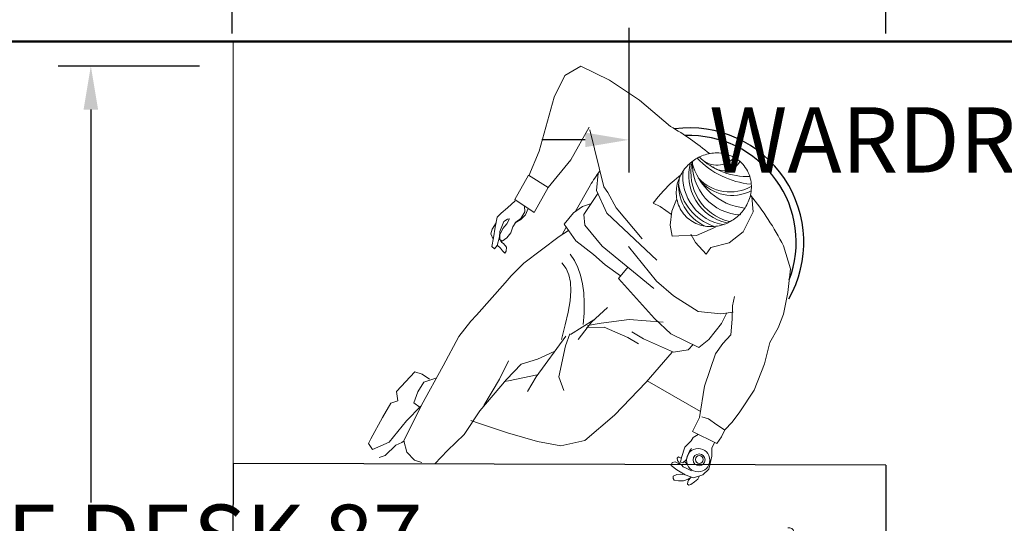
# Model space of a CAD drawing. Units: inches. Extents: x -466983 to 1020, y 324 to 318697.
# Tile 39 of 97: x 817 to 908, y 781 to 827. Entities that reach past the tile are written whole.
import ezdxf

# ---------------------------------------------------------------- set-up
doc = ezdxf.new("R2010")
doc.units = ezdxf.units.IN
doc.header["$MEASUREMENT"] = 0
for name, color, linetype, lineweight in [('A-ANNO-DIMS', 2, 'Continuous', 18), ('A-FLOR-PATT', 252, 'Continuous', 13), ('A-FURN', 8, 'Continuous', 18), ('A-WALL', 7, 'Continuous', 50), ('CBV_01', 7, 'Continuous', 0)]:
    doc.layers.add(name, color=color, linetype=linetype, lineweight=lineweight)
doc.layers.add('Office Desk', color=30, linetype='Continuous', true_color=0xeb7500)
doc.styles.get("Standard").update_dxf_attribs({"font": 'arial.ttf'})
doc.dimstyles.get("Standard").update_dxf_attribs({"dimtxt": 6, "dimasz": 4, "dimexe": 3, "dimexo": 3, "dimgap": 0.09, "dimtad": 0, "dimtih": 1, "dimtoh": 1, "dimdec": 1, "dimzin": 0, "dimdsep": 46, "dimlunit": 3, "dimtxsty": 'Standard', "dimcen": 0.09, "dimadec": 0, "dimazin": 0, "dimtfac": 1, "dimtdec": 1, "dimtofl": 0, "dimtmove": 0, "dimatfit": 3, "dimfxl": 1, "dimtolj": 1, "dimtzin": 0, "dimarcsym": 0})

# ---------------------------------------------------------------- blocks, each defined once
blk = doc.blocks.new('Offce Table')
at = {"layer": 'CBV_01'}
h = blk.add_hatch(dxfattribs=at)
h.set_pattern_fill('HEX', color=256, scale=1.206041, angle=-45.15377, style=0)
h.set_pattern_definition([(44.846232, (2370.5468, 299.66597), (0.18414034, -0.18513138), [0.1507551, -0.30151019]), (284.846232, (2370.5468, 299.66597), (-0.25239865, -0.06690453), [0.1507551, -0.30151019]), (344.846232, (2370.6537, 299.77229), (-0.06825831, -0.25203591), [0.1507551, -0.30151019])])
h.paths.add_polyline_path([(2601.472, 956.599), (2601.473, 957.136, -4.924372), (2599.622, 957.141), (2599.621, 956.604, 3.823416)])
for p, q in [((2608.415, 1012.503, -0.016), (2606.746, 1009.522, -0.016)), ((2609.784, 1007.023, -0.016), (2608.49, 1012.271, -0.016)), ((2606.746, 1009.522, -0.016), (2604.659, 1006.977, -0.016)), ((2609.256, 1008.271, -0.016), (2609.109, 1006.706, -0.016)), ((2602.849, 1008.103, -0.016), (2601.613, 1005.868, -0.016)), ((2604.659, 1006.977, -0.016), (2602.849, 1008.103, -0.016)), ((2604.659, 1006.977, -0.016), (2603.369, 1004.683, -0.016)), ((2607.133, 1004.729, -0.016), (2608.517, 1007.151, -0.016)), ((2609.109, 1006.706, -0.016), (2610.057, 1004.601, -0.016)), ((2603.369, 1004.683, -0.016), (2601.613, 1005.868, -0.016)), ((2610.057, 1004.601, -0.016), (2614.644, 1000.305, -0.016)), ((2605.941, 1002.644, -0.016), (2606.327, 1003.319, -0.016)), ((2612.11, 994.853, -0.016), (2609.52, 994.501, -0.016)), ((2615.216, 994.607, -0.016), (2612.11, 994.853, -0.016)), ((2609.52, 994.501, -0.016), (2608.271, 994.303, -0.016)), ((2618.647, 986.395, -0.016), (2613.748, 989.194, -0.016)), ((2625.938, 974.583, -0.016), (2624.545, 974.304, -0.016)), ((2626.476, 972.945, -0.016), (2617.003, 972.971, -0.016)), ((2616.528, 972.498, -0.016), (2616.499, 961.604, -0.016)), ((2617.001, 972.023, -0.016), (2616.976, 963.024, -0.016)), ((2622.832, 972.481, -0.016), (2617.475, 972.496, -0.016)), ((2622.49, 972.008, -0.016), (2617.948, 972.021, -0.016)), ((2626.001, 972.473, -0.016), (2622.97, 972.481, -0.016)), ((2625.552, 972, -0.016), (2623.065, 972.007, -0.016)), ((2623.609, 963.48, -0.016), (2623.632, 972.005, -0.016)), ((2626.919, 961.576, -0.016), (2626.948, 972.47, -0.016)), ((2590.067, 965.862, -0.016), (2590.368, 971.161, -0.016)), ((2590.877, 971.137, -0.016), (2603.66, 971.102, -0.016)), ((2591.166, 971.955, -0.016), (2608.412, 971.908, -0.016)), ((2591.557, 971.135, -0.016), (2591.555, 970.498, -0.016)), ((2592.439, 971.132, -0.016), (2592.437, 970.496, -0.016)), ((2593.31, 971.13, -0.016), (2593.309, 970.493, -0.016)), ((2600.28, 971.111, -0.016), (2600.278, 970.474, -0.016)), ((2601.151, 971.109, -0.016), (2601.15, 970.472, -0.016)), ((2602.023, 971.107, -0.016), (2602.021, 970.47, -0.016)), ((2602.894, 971.104, -0.016), (2602.892, 970.467, -0.016)), ((2604.302, 971.1, -0.016), (2606.269, 971.095, -0.016)), ((2609.478, 965.81, -0.016), (2609.206, 971.11, -0.016)), ((2617.473, 971.548, -0.016), (2617.451, 963.496, -0.016)), ((2622.661, 963.482, -0.016), (2622.684, 971.877, -0.016)), ((2625.977, 963.473, -0.016), (2625.998, 971.525, -0.016)), ((2626.449, 962.998, -0.016), (2626.473, 971.998, -0.016)), ((2590.761, 970.595, -0.016), (2590.787, 971.051, -0.016)), ((2590.827, 970.256, -0.016), (2603.657, 970.221, -0.016)), ((2590.851, 970.5, -0.016), (2603.658, 970.465, -0.016)), ((2592.1, 970.252, -0.016), (2592.098, 969.616, -0.016)), ((2592.971, 970.25, -0.016), (2592.97, 969.613, -0.016)), ((2593.842, 970.248, -0.016), (2593.841, 969.611, -0.016)), ((2594.714, 970.245, -0.016), (2594.712, 969.609, -0.016)), ((2595.585, 970.243, -0.016), (2595.583, 969.606, -0.016)), ((2596.456, 970.241, -0.016), (2596.454, 969.604, -0.016)), ((2597.327, 970.238, -0.016), (2597.326, 969.602, -0.016)), ((2598.199, 970.236, -0.016), (2598.197, 969.599, -0.016)), ((2599.07, 970.234, -0.016), (2599.068, 969.597, -0.016)), ((2599.941, 970.231, -0.016), (2599.939, 969.595, -0.016)), ((2600.812, 970.229, -0.016), (2600.811, 969.592, -0.016)), ((2601.683, 970.227, -0.016), (2601.682, 969.59, -0.016)), ((2603.75, 971.012, -0.016), (2603.749, 970.555, -0.016)), ((2604.211, 971.011, -0.016), (2604.21, 970.554, -0.016)), ((2604.3, 970.464, -0.016), (2606.267, 970.458, -0.016)), ((2604.928, 971.099, -0.016), (2604.926, 970.462, -0.016)), ((2605.015, 970.218, -0.016), (2605.551, 970.216, -0.016)), ((2605.643, 971.097, -0.016), (2605.642, 970.46, -0.016)), ((2606.359, 971.005, -0.016), (2606.358, 970.548, -0.016)), ((2606.821, 971.004, -0.016), (2606.82, 970.547, -0.016)), ((2606.909, 970.213, -0.016), (2608.289, 970.209, -0.016)), ((2606.91, 970.457, -0.016), (2608.29, 970.453, -0.016)), ((2606.911, 971.093, -0.016), (2608.697, 971.089, -0.016)), ((2607.309, 970.212, -0.016), (2607.307, 969.575, -0.016)), ((2607.311, 971.092, -0.016), (2607.31, 970.456, -0.016)), ((2607.799, 970.21, -0.016), (2607.798, 969.573, -0.016)), ((2607.802, 971.091, -0.016), (2607.8, 970.454, -0.016)), ((2608.292, 971.09, -0.016), (2608.288, 969.572, -0.016)), ((2608.855, 969.666, -0.016), (2608.787, 971.003, -0.016)), ((2590.711, 969.714, -0.016), (2590.737, 970.171, -0.016)), ((2590.777, 969.375, -0.016), (2603.655, 969.34, -0.016)), ((2590.801, 969.619, -0.016), (2603.656, 969.585, -0.016)), ((2591.215, 969.374, -0.016), (2591.214, 968.737, -0.016)), ((2592.098, 969.371, -0.016), (2592.096, 968.735, -0.016)), ((2592.969, 969.369, -0.016), (2592.967, 968.732, -0.016)), ((2593.84, 969.367, -0.016), (2593.838, 968.73, -0.016)), ((2594.711, 969.364, -0.016), (2594.71, 968.728, -0.016)), ((2595.583, 969.362, -0.016), (2595.581, 968.725, -0.016)), ((2596.454, 969.36, -0.016), (2596.452, 968.723, -0.016)), ((2597.325, 969.357, -0.016), (2597.323, 968.721, -0.016)), ((2598.196, 969.355, -0.016), (2598.195, 968.718, -0.016)), ((2599.067, 969.353, -0.016), (2599.066, 968.716, -0.016)), ((2599.939, 969.35, -0.016), (2599.937, 968.714, -0.016)), ((2600.81, 969.348, -0.016), (2600.808, 968.711, -0.016)), ((2601.681, 969.346, -0.016), (2601.679, 968.709, -0.016)), ((2602.552, 969.343, -0.016), (2602.55, 968.463, -0.016)), ((2603.747, 970.131, -0.016), (2603.746, 969.675, -0.016)), ((2604.925, 970.128, -0.016), (2604.924, 969.671, -0.016)), ((2605.014, 969.581, -0.016), (2605.549, 969.579, -0.016)), ((2605.641, 970.126, -0.016), (2605.64, 969.669, -0.016)), ((2606.818, 970.123, -0.016), (2606.817, 969.666, -0.016)), ((2606.907, 969.576, -0.016), (2608.765, 969.571, -0.016)), ((2606.907, 969.332, -0.016), (2608.787, 969.327, -0.016)), ((2607.307, 969.331, -0.016), (2607.305, 968.694, -0.016)), ((2607.797, 969.329, -0.016), (2607.795, 968.693, -0.016)), ((2608.287, 969.328, -0.016), (2608.283, 967.81, -0.016)), ((2590.611, 967.953, -0.016), (2590.637, 968.409, -0.016)), ((2590.661, 968.834, -0.016), (2590.687, 969.29, -0.016)), ((2590.727, 968.494, -0.016), (2602.55, 968.463, -0.016)), ((2590.751, 968.738, -0.016), (2602.551, 968.707, -0.016)), ((2591.751, 968.491, -0.016), (2591.75, 967.855, -0.016)), ((2592.623, 968.489, -0.016), (2592.621, 967.852, -0.016)), ((2593.494, 968.487, -0.016), (2593.492, 967.85, -0.016)), ((2594.365, 968.484, -0.016), (2594.363, 967.848, -0.016)), ((2595.236, 968.482, -0.016), (2595.235, 967.845, -0.016)), ((2596.108, 968.48, -0.016), (2596.106, 967.843, -0.016)), ((2596.979, 968.477, -0.016), (2596.977, 967.841, -0.016)), ((2597.85, 968.475, -0.016), (2597.848, 967.838, -0.016)), ((2598.721, 968.473, -0.016), (2598.719, 967.836, -0.016)), ((2599.592, 968.47, -0.016), (2599.591, 967.834, -0.016)), ((2600.464, 968.468, -0.016), (2600.462, 967.831, -0.016)), ((2601.335, 968.466, -0.016), (2601.333, 967.829, -0.016)), ((2602.092, 968.464, -0.016), (2602.091, 967.827, -0.016)), ((2603.745, 969.25, -0.016), (2603.741, 967.913, -0.016)), ((2604.295, 968.458, -0.016), (2606.262, 968.453, -0.016)), ((2604.92, 968.456, -0.016), (2604.919, 967.819, -0.016)), ((2605.636, 968.454, -0.016), (2605.635, 967.817, -0.016)), ((2606.816, 969.242, -0.016), (2606.815, 968.785, -0.016)), ((2606.904, 968.451, -0.016), (2608.285, 968.447, -0.016)), ((2606.905, 968.695, -0.016), (2608.285, 968.691, -0.016)), ((2607.304, 968.45, -0.016), (2607.303, 967.813, -0.016)), ((2607.794, 968.448, -0.016), (2607.793, 967.812, -0.016)), ((2608.946, 967.904, -0.016), (2608.877, 969.241, -0.016)), ((2590.561, 967.072, -0.016), (2590.587, 967.528, -0.016)), ((2590.677, 967.613, -0.016), (2603.65, 967.579, -0.016)), ((2590.701, 967.858, -0.016), (2603.651, 967.823, -0.016)), ((2591.526, 967.611, -0.016), (2591.525, 966.974, -0.016)), ((2592.409, 967.609, -0.016), (2592.407, 966.972, -0.016)), ((2593.28, 967.606, -0.016), (2593.278, 966.97, -0.016)), ((2594.151, 967.604, -0.016), (2594.149, 966.967, -0.016)), ((2595.022, 967.602, -0.016), (2595.021, 966.965, -0.016)), ((2595.893, 967.599, -0.016), (2595.892, 966.963, -0.016)), ((2596.765, 967.597, -0.016), (2596.763, 966.96, -0.016)), ((2597.636, 967.595, -0.016), (2597.634, 966.958, -0.016)), ((2598.507, 967.592, -0.016), (2598.505, 966.956, -0.016)), ((2599.378, 967.59, -0.016), (2599.377, 966.953, -0.016)), ((2600.25, 967.588, -0.016), (2600.248, 966.951, -0.016)), ((2601.121, 967.585, -0.016), (2601.119, 966.949, -0.016)), ((2601.992, 967.583, -0.016), (2601.99, 966.946, -0.016)), ((2602.863, 967.581, -0.016), (2602.862, 966.944, -0.016)), ((2603.74, 967.488, -0.016), (2603.739, 967.032, -0.016)), ((2604.202, 967.487, -0.016), (2604.201, 967.031, -0.016)), ((2604.204, 968.368, -0.016), (2604.203, 967.911, -0.016)), ((2604.292, 967.577, -0.016), (2606.26, 967.572, -0.016)), ((2604.293, 967.821, -0.016), (2606.26, 967.816, -0.016)), ((2604.918, 967.575, -0.016), (2604.916, 966.938, -0.016)), ((2605.634, 967.573, -0.016), (2605.632, 966.937, -0.016)), ((2606.352, 968.362, -0.016), (2606.351, 967.906, -0.016)), ((2606.814, 968.361, -0.016), (2606.813, 967.904, -0.016)), ((2606.902, 967.814, -0.016), (2608.855, 967.809, -0.016)), ((2606.902, 967.57, -0.016), (2608.878, 967.565, -0.016)), ((2607.302, 967.569, -0.016), (2607.3, 966.932, -0.016)), ((2607.792, 967.568, -0.016), (2607.79, 966.931, -0.016)), ((2608.282, 967.566, -0.016), (2608.281, 966.929, -0.016)), ((2610.991, 968.125, -0.016), (2610.989, 967.24, -0.016)), ((2613.126, 967.234, -0.016), (2613.129, 968.12, -0.016)), ((2618.946, 967.738, -0.016), (2618.938, 964.699, -0.016)), ((2621.142, 967.732, -0.016), (2618.946, 967.738, -0.016)), ((2621.134, 964.693, -0.016), (2621.142, 967.732, -0.016)), ((2590.651, 966.977, -0.016), (2603.649, 966.942, -0.016)), ((2604.291, 966.94, -0.016), (2606.258, 966.935, -0.016)), ((2606.35, 967.481, -0.016), (2606.348, 967.025, -0.016)), ((2606.811, 967.48, -0.016), (2606.81, 967.024, -0.016)), ((2606.9, 966.933, -0.016), (2608.901, 966.928, -0.016)), ((2608.991, 967.023, -0.016), (2608.968, 967.479, -0.016)), ((2590.463, 965.974, -0.016), (2590.489, 966.43, -0.016)), ((2590.553, 965.879, -0.016), (2603.646, 965.843, -0.016)), ((2590.579, 966.515, -0.016), (2603.647, 966.48, -0.016)), ((2591.208, 966.514, -0.016), (2591.206, 965.877, -0.016)), ((2592.09, 966.511, -0.016), (2592.088, 965.874, -0.016)), ((2592.961, 966.509, -0.016), (2592.959, 965.872, -0.016)), ((2593.832, 966.507, -0.016), (2593.831, 965.87, -0.016)), ((2594.704, 966.504, -0.016), (2594.702, 965.867, -0.016)), ((2595.575, 966.502, -0.016), (2595.573, 965.865, -0.016)), ((2596.446, 966.5, -0.016), (2596.444, 965.863, -0.016)), ((2597.317, 966.497, -0.016), (2597.316, 965.86, -0.016)), ((2598.189, 966.495, -0.016), (2598.187, 965.858, -0.016)), ((2599.06, 966.493, -0.016), (2599.058, 965.856, -0.016)), ((2599.931, 966.49, -0.016), (2599.929, 965.853, -0.016)), ((2600.802, 966.488, -0.016), (2600.8, 965.851, -0.016)), ((2601.673, 966.485, -0.016), (2601.672, 965.849, -0.016)), ((2602.545, 966.483, -0.016), (2602.543, 965.846, -0.016)), ((2603.737, 966.39, -0.016), (2603.736, 965.933, -0.016)), ((2604.199, 966.389, -0.016), (2604.198, 965.932, -0.016)), ((2604.288, 965.842, -0.016), (2606.255, 965.836, -0.016)), ((2604.289, 966.478, -0.016), (2606.257, 966.473, -0.016)), ((2604.915, 966.477, -0.016), (2604.913, 965.84, -0.016)), ((2605.631, 966.475, -0.016), (2605.629, 965.838, -0.016)), ((2606.347, 966.383, -0.016), (2606.346, 965.926, -0.016)), ((2591.651, 963.61, -0.016), (2591.652, 964.18, -0.016)), ((2591.652, 964.18, -0.016), (2607.884, 964.136, -0.016)), ((2607.883, 963.567, -0.016), (2607.884, 964.136, -0.016)), ((2618.938, 964.699, -0.016), (2621.134, 964.693, -0.016)), ((2591.651, 963.61, -0.016), (2607.883, 963.567, -0.016)), ((2617.924, 963.021, -0.016), (2622.186, 963.01, -0.016)), ((2624.081, 963.005, -0.016), (2625.502, 963.001, -0.016)), ((2617.449, 962.549, -0.016), (2625.974, 962.526, -0.016)), ((2616.971, 961.129, -0.016), (2626.444, 961.104, -0.016)), ((2587.523, 957.485, -0.016), (2587.529, 959.809, -0.016)), ((2588.012, 959.808, -0.016), (2587.529, 959.809, -0.016)), ((2588.008, 958.361, -0.016), (2588.012, 959.808, -0.016)), ((2613.097, 959.741, -0.016), (2588.012, 959.808, -0.016)), ((2613.093, 958.293, -0.016), (2613.097, 959.741, -0.016)), ((2613.097, 959.741, -0.016), (2613.58, 959.739, -0.016)), ((2613.574, 957.415, -0.016), (2613.58, 959.739, -0.016)), ((2613.575, 957.83, -0.016), (2587.524, 957.9, -0.016)), ((2613.093, 958.293, -0.016), (2588.008, 958.361, -0.016)), ((2613.574, 957.415, -0.016), (2587.523, 957.485, -0.016)), ((2599.623, 957.453, -0.016), (2599.616, 954.956, -0.016)), ((2601.467, 954.951, -0.016), (2601.474, 957.448, -0.016))]:
    blk.add_line(p, q, dxfattribs=at)
at = {"layer": 'CBV_01', "elevation": -0.016}
for points in [[(2615.905, 1012.577), (2613.053, 1014.982), (2610.299, 1016.845), (2607.657, 1018.131), (2606.194, 1017.275), (2605.217, 1015.268), (2603.853, 1010.314), (2602.879, 1008.045)], [(2615.988, 1004.478), (2614.96, 1005.208), (2614.308, 1005.525), (2614.757, 1006.113), (2615.264, 1006.672), (2615.861, 1007.303), (2616.828, 1008.098)], [(2609.237, 1006.422), (2607.928, 1004.486), (2608.031, 1003.515), (2609.627, 1001.587), (2614.38, 997.692)], [(2609.784, 1007.023), (2610.157, 1006.5), (2610.923, 1005.091), (2613.301, 1002.25)], [(2601.645, 1005.757), (2600.928, 1005.093), (2600.35, 1004.604), (2599.991, 1004.244), (2599.803, 1003.315), (2599.638, 1002.347), (2599.483, 1001.54), (2599.724, 1001.344), (2599.967, 1001.637), (2600.182, 1002.428), (2600.223, 1002.939), (2600.601, 1003.849), (2600.919, 1004.057), (2601.126, 1004.099), (2600.864, 1003.615), (2600.488, 1003.194), (2600.232, 1002.61), (2600.215, 1002.19), (2600.434, 1002.033), (2600.876, 1002.337), (2601.229, 1002.797), (2601.417, 1003.366), (2601.693, 1003.781), (2602.143, 1004.116), (2602.508, 1004.736), (2602.488, 1005.264)], [(2611.311, 998.838), (2609.891, 999.854), (2608.816, 1000.825), (2607.213, 1002.053), (2606.132, 1003.597), (2607.005, 1004.637), (2607.817, 1005.219), (2608.551, 1005.472)], [(2620.03, 1003.316), (2618.279, 1002.557), (2616.657, 1002.54), (2616.056, 1002.487), (2615.859, 1003.504), (2616.03, 1004.802), (2616.435, 1005.872)], [(2623.369, 1006.108), (2623.489, 1004.742), (2622.583, 1002.88), (2621.297, 1001.894), (2619.588, 1001.46), (2619.177, 1000.853), (2618.193, 1001.908), (2617.768, 1002.691)], [(2602.82, 1005.043), (2602.594, 1004.451), (2602.149, 1004.017), (2601.646, 1003.729)], [(2599.88, 1003.719), (2599.524, 1003.13), (2599.408, 1002.704), (2599.605, 1002.226)], [(2606.528, 1003.032), (2605.68, 1002.471), (2602.418, 1000.03), (2601.273, 998.86), (2600.724, 998.206)], [(2599.975, 1001.667), (2600.29, 1001.386), (2600.484, 1001.137), (2600.694, 1000.949), (2600.805, 1001.115), (2600.843, 1001.497), (2600.575, 1001.831), (2600.401, 1001.911), (2600.29, 1002.105)], [(2621.645, 995.508), (2620.535, 995.357), (2618.448, 995.567), (2616.162, 997.025), (2614.619, 998.351), (2612.039, 1001.547)], [(2626.275, 1001.616), (2626.928, 999.499), (2626.674, 997.32), (2626.279, 995.325), (2625.783, 994.07), (2625.011, 992.719), (2624.523, 990.769), (2623.577, 988.351), (2622.255, 986.346), (2621.571, 985.413), (2620.884, 984.711), (2620.567, 984.06), (2620.156, 983.454), (2617.921, 984.542), (2618.555, 985.845), (2619.033, 988.72), (2620.019, 991.694), (2620.704, 992.627), (2621.436, 993.422), (2621.56, 994.859), (2621.592, 996.109), (2621.768, 996.945)], [(2621.045, 995.403), (2620.596, 994.482), (2619.433, 993.012), (2618.508, 992.282), (2615.939, 993.532), (2614.417, 994.924), (2611.117, 998.606), (2612.006, 999.68)], [(2598.079, 995.226), (2600.724, 998.206)], [(2610.106, 995.943), (2608.639, 994.585), (2607.406, 992.997)], [(2593.057, 981.705), (2592.391, 981.926), (2591.699, 982.654), (2591.425, 983.702), (2593.018, 986.977), (2595.029, 990.571), (2596.471, 993.266), (2597.559, 994.696), (2598.079, 995.226)], [(2608.868, 994.819), (2606.706, 993.453)], [(2612.969, 992.593), (2611.989, 993.184), (2609.802, 994.134), (2608.181, 994.117)], [(2606.3, 993.316), (2603.556, 989.557), (2602.782, 988.235)], [(2606.666, 993.53), (2606.258, 992.422), (2605.658, 989.579), (2606.092, 988.322)], [(2617.981, 992.539), (2617.509, 992.046), (2616.173, 991.839), (2613.427, 993.06), (2612.354, 993.697)], [(2616.041, 991.842), (2613.653, 989.084), (2610.743, 986.059), (2608.035, 983.719), (2605.833, 983.223), (2603.674, 983.62), (2600.931, 984.432), (2598.346, 985.299), (2597.555, 985.553)], [(2601.016, 991.054), (2600.194, 989.364), (2598.749, 986.932)], [(2602.176, 990.751), (2603.695, 991.187), (2605.212, 991.886)], [(2602.176, 990.751), (2600.825, 989.318), (2598.386, 986.455), (2596.938, 984.285), (2595.43, 982.798), (2594.268, 981.566)], [(2593.781, 989.349), (2593.092, 989.815), (2592.407, 990.018), (2590.745, 988.214), (2590.859, 987.374), (2590.231, 987.158), (2589.457, 985.836), (2588.374, 983.881), (2588.169, 983.458), (2588.543, 982.884), (2590.06, 983.583), (2591.668, 985.544), (2592.967, 986.871)], [(2594.358, 989.46), (2593.258, 989.081), (2592.69, 988.182), (2592.333, 987.18), (2592.916, 986.765)], [(2603.658, 989.768), (2602.347, 989.491), (2601.036, 989.215), (2600.616, 989.158)], [(2620.869, 984.711), (2620.142, 985.171), (2619.396, 985.724), (2618.764, 985.904)], [(2618.427, 984.285), (2617.992, 984.009), (2617.799, 983.689), (2617.455, 983.369), (2617.216, 983.109), (2616.915, 982.152), (2616.829, 981.743), (2617.026, 981.685), (2617.34, 981.945), (2617.643, 982.751), (2617.837, 982.995)], [(2589.13, 982.155), (2589.704, 982.337), (2590.671, 983.296), (2591.214, 983.532), (2591.428, 983.678)], [(2619.946, 983.546), (2619.695, 983.03), (2619.703, 982.275), (2619.429, 981.094), (2618.876, 980.574), (2618.018, 980.278), (2617.259, 980.573), (2616.468, 981.032), (2615.95, 981.435), (2616.038, 981.692), (2616.339, 981.771), (2616.582, 981.653), (2616.932, 981.445), (2617.054, 981.31), (2617.389, 981.148), (2617.632, 981.03), (2617.814, 980.941)], [(2616.879, 982.095), (2616.619, 982.222), (2616.509, 982.091), (2616.53, 981.897), (2616.727, 981.641), (2616.83, 981.522)], [(2617.45, 981.473), (2617.29, 981.711), (2617.159, 981.821)], [(2617.842, 980.339), (2617.529, 980.17), (2617.087, 980.017), (2616.633, 980.031), (2616.226, 980.091), (2616.132, 980.229), (2616.139, 980.433), (2616.479, 980.612), (2616.793, 980.643), (2616.96, 980.608), (2617.219, 980.62)], [(2618.571, 980.467), (2618.408, 980.179), (2618.096, 979.917), (2617.756, 979.691), (2617.581, 979.616), (2617.451, 979.725), (2617.476, 979.92), (2617.558, 980.087), (2617.731, 980.301)], [(2612.055, 966.169), (2611.856, 964.989), (2611.679, 963.716), (2611.02, 962.076), (2610.22, 960.793), (2609.486, 959.75)], [(2606.891, 963.569), (2606.795, 962.987), (2606.508, 962.105), (2606.218, 960.599), (2605.987, 959.76)], [(2605.259, 957.437), (2604.573, 956.5), (2603.741, 956.009), (2602.914, 954.947)], [(2607.854, 957.43), (2607.669, 957.168), (2607.117, 956.845), (2606.434, 956.343), (2605.915, 956.117), (2604.644, 955.241), (2604.076, 954.87), (2602.914, 954.897)]]:
    blk.add_lwpolyline(points, dxfattribs=at)
blk.add_lwpolyline([(2617.847, 1009.329, -0.080167), (2618.927, 1009.931, -0.088923), (2620.168, 1010.146, -0.104957), (2621.517, 1009.851, -0.120011), (2622.66, 1008.958, -0.120011), (2623.265, 1007.64, -0.104957), (2623.24, 1006.259, -0.088923), (2622.744, 1005.101, -0.080167), (2621.908, 1004.19, -0.080167), (2620.828, 1003.587, -0.088923), (2619.587, 1003.373, -0.104957), (2618.238, 1003.667, -0.120011), (2617.095, 1004.56, -0.120011), (2616.491, 1005.879, -0.104957), (2616.516, 1007.26, -0.088923), (2617.012, 1008.417, -0.080167)], format="xyb", close=True, dxfattribs=at)
at = {"layer": 'CBV_01'}
for points in [[(2605.883, 992.996), (2606.24, 994.337), (2606.508, 995.522), (2606.681, 996.562), (2606.754, 997.472), (2606.719, 998.261), (2606.572, 998.944), (2606.304, 999.532), (2605.911, 1000.037)], [(2607.865, 994.383), (2607.958, 995.416), (2607.981, 996.384), (2607.937, 997.288), (2607.824, 998.126), (2607.643, 998.9), (2607.394, 999.61), (2607.076, 1000.254), (2606.691, 1000.834)]]:
    blk.add_lwpolyline(points, dxfattribs=at)
at = {"layer": 'CBV_01', "elevation": -0.016}
for points in [[(2622.965, 972.508), (2622.413, 972.397), (2622.523, 971.845), (2623.075, 971.955)], [(2618.41, 970.567), (2617.848, 970.568), (2617.846, 970.005), (2618.409, 970.004)], [(2619.358, 970.564), (2618.795, 970.566), (2618.794, 970.003), (2619.356, 970.001)], [(2620.305, 970.562), (2619.742, 970.563), (2619.741, 970), (2620.304, 969.999)], [(2621.252, 970.559), (2620.69, 970.561), (2620.688, 969.998), (2621.251, 969.996)], [(2618.408, 969.54), (2617.845, 969.541), (2617.843, 968.978), (2618.406, 968.977)], [(2619.355, 969.537), (2618.792, 969.539), (2618.791, 968.976), (2619.353, 968.974)], [(2620.302, 969.535), (2619.74, 969.536), (2619.738, 968.973), (2620.301, 968.972)], [(2621.25, 969.532), (2620.687, 969.534), (2620.685, 968.971), (2621.248, 968.969)], [(2622.197, 969.53), (2621.634, 969.531), (2621.633, 968.968), (2622.195, 968.967)], [(2619.597, 967.597), (2619.034, 967.599), (2619.032, 967.036), (2619.595, 967.034)], [(2620.292, 967.595), (2619.73, 967.597), (2619.728, 967.034), (2620.291, 967.032)], [(2620.988, 967.594), (2620.425, 967.595), (2620.424, 967.032), (2620.986, 967.031)], [(2619.595, 966.902), (2619.032, 966.904), (2619.031, 966.341), (2619.593, 966.339)], [(2620.29, 966.9), (2619.728, 966.902), (2619.726, 966.339), (2620.289, 966.337)], [(2620.986, 966.898), (2620.423, 966.9), (2620.422, 966.337), (2620.985, 966.335)], [(2619.593, 966.207), (2619.03, 966.208), (2619.029, 965.645), (2619.591, 965.644)], [(2620.289, 966.205), (2619.726, 966.207), (2619.724, 965.643), (2620.287, 965.642)], [(2620.984, 966.203), (2620.422, 966.205), (2620.42, 965.642), (2620.983, 965.64)], [(2619.591, 965.475), (2619.028, 965.477), (2619.027, 964.914), (2619.589, 964.912)], [(2620.287, 965.473), (2619.724, 965.475), (2619.722, 964.912), (2620.285, 964.91)], [(2620.982, 965.471), (2620.42, 965.473), (2620.418, 964.91), (2620.981, 964.908)], [(2624.959, 963.21), (2624.96, 963.66), (2624.678, 963.661), (2624.677, 963.211)]]:
    blk.add_lwpolyline(points, close=True, dxfattribs=at)
at = {"layer": 'CBV_01', "const_width": 0.0942, "elevation": -0.016}
blk.add_lwpolyline([(2624.828, 963.196, -0.40574), (2623.816, 960.526, -1.618522), (2623.611, 961.83, -1.478802), (2622.602, 960.078, -0.24273), (2622.249, 961.227, -0.24273)], format="xyb", dxfattribs=at)
at = {"layer": 'CBV_01'}
for centre, radius in [((2618.438, 981.914, -0.016), 1.073), ((2618.528, 981.945, -0.016), 0.545), ((2618.543, 981.975, -0.016), 0.359), ((2607.595, 966.107, -0.016), 0.106), ((2608.057, 966.106, -0.016), 0.106), ((2608.519, 966.105, -0.016), 0.106), ((2594.113, 965.106, -0.016), 0.106), ((2594.575, 965.104, -0.016), 0.106), ((2595.037, 965.103, -0.016), 0.106), ((2595.499, 965.102, -0.016), 0.106), ((2595.961, 965.101, -0.016), 0.106), ((2596.423, 965.099, -0.016), 0.106), ((2596.885, 965.098, -0.016), 0.106)]:
    blk.add_circle(centre, radius, dxfattribs=at)
for centre, radius, start, end in [((2602.197, 989.221, -0.016), 27.082, 50.37515, 59.59099), ((2622.039, 1008.072, -0.016), 4.456, 164.47486, 257.30647), ((2622.408, 1008.336, -0.016), 4.634, 167.21461, 256.32515), ((2623.354, 1010.71, -0.016), 5.667, 194.03684, 263.23405), ((2622.533, 1009.067, -0.016), 4.614, 175.94557, 267.66665), ((2623.978, 1014.99, -0.016), 7.744, 223.41938, 264.68964), ((2622.956, 1014.334, -0.016), 6.357, 225.72213, 272.27484), ((2620.166, 1011.122, -0.016), 2.108, 227.18188, 318.83431), ((2620.826, 1010.16, -0.016), 1.655, 231.54376, 331.05244), ((2617.636, 1001.94, -0.016), 10.504, 141.43972, 150.25259), ((2621.493, 1007.946, -0.016), 4.465, 172.97935, 261.42536), ((2620.734, 1007.169, -0.016), 4.09, 171.47064, 246.35242), ((2621.463, 1008.017, -0.016), 4.872, 188.62106, 250.62094), ((2621.377, 1010.531, -0.016), 3.975, 222.55221, 299.84347), ((2621.553, 1010.092, -0.016), 3.854, 219.71778, 296.81649), ((2602.197, 989.221, -0.016), 27.082, 27.2384, 39.00595), ((2626.774, 975.233, -0.016), 0.474, 11.29645, 101.29645), ((2626.403, 974.675, -0.016), 0.474, 11.29645, 101.29645), ((2622.78, 973.469, -0.016), 0.474, 11.29645, 101.29645), ((2624.638, 973.84, -0.016), 0.474, 101.29645, 191.29645), ((2626.031, 974.118, -0.016), 0.474, 11.29645, 101.29645), ((2617.002, 972.497, -0.016), 0.474, 89.84532, 179.84532), ((2617.474, 972.022, -0.016), 0.474, 89.84532, 179.84532), ((2617.947, 971.547, -0.016), 0.474, 89.84532, 179.84532), ((2591.164, 971.159, -0.016), 0.796, 89.84623, 179.84623), ((2590.877, 971.046, -0.016), 0.0902, 89.84623, 176.75215), ((2603.66, 971.012, -0.016), 0.0902, 359.84623, 89.84623), ((2604.302, 971.01, -0.016), 0.0902, 89.84623, 179.84623), ((2608.41, 971.112, -0.016), 0.796, 359.84623, 89.84623), ((2590.827, 970.166, -0.016), 0.0902, 89.84623, 176.75215), ((2590.851, 970.59, -0.016), 0.0902, 176.75215, 269.84623), ((2603.657, 970.131, -0.016), 0.0902, 359.84623, 89.84623), ((2603.658, 970.556, -0.016), 0.0902, 269.84623, 359.84623), ((2604.3, 970.554, -0.016), 0.0902, 179.84623, 269.84623), ((2605.015, 970.127, -0.016), 0.0902, 89.84623, 179.84623), ((2605.551, 970.126, -0.016), 0.0902, 359.84623, 89.84623), ((2606.268, 970.549, -0.016), 0.0902, 269.84623, 359.84623), ((2606.269, 971.005, -0.016), 0.0902, 359.84623, 89.84623), ((2606.909, 970.122, -0.016), 0.0902, 89.84623, 179.84623), ((2606.91, 970.547, -0.016), 0.0902, 179.84623, 269.84623), ((2606.911, 971.003, -0.016), 0.0902, 89.84623, 179.84623), ((2608.696, 970.998, -0.016), 0.0902, 2.94029, 89.84623), ((2590.777, 969.285, -0.016), 0.0902, 89.84623, 176.75215), ((2590.801, 969.709, -0.016), 0.0902, 176.75215, 269.84623), ((2603.655, 969.25, -0.016), 0.0902, 359.84623, 89.84623), ((2603.656, 969.675, -0.016), 0.0902, 269.84623, 359.84623), ((2605.014, 969.671, -0.016), 0.0902, 179.84623, 269.84623), ((2605.549, 969.67, -0.016), 0.0902, 269.84623, 359.84623), ((2606.906, 969.241, -0.016), 0.0902, 89.84623, 179.84623), ((2606.907, 969.666, -0.016), 0.0902, 179.84623, 269.84623), ((2608.765, 969.661, -0.016), 0.0902, 269.84623, 2.94029), ((2608.787, 969.236, -0.016), 0.0902, 2.94029, 89.84623), ((2590.727, 968.404, -0.016), 0.0902, 89.84623, 176.75215), ((2590.751, 968.828, -0.016), 0.0902, 176.75215, 269.84623), ((2604.295, 968.368, -0.016), 0.0902, 89.84623, 179.84623), ((2606.262, 968.362, -0.016), 0.0902, 359.84623, 89.84623), ((2606.904, 968.361, -0.016), 0.0902, 89.84623, 179.84623), ((2606.905, 968.785, -0.016), 0.0902, 179.84623, 269.84623), ((2612.06, 968.122, -0.016), 1.069, 335.38444, 204.30803), ((2590.677, 967.523, -0.016), 0.0902, 89.84623, 176.75215), ((2590.701, 967.948, -0.016), 0.0902, 176.75215, 269.84623), ((2603.65, 967.488, -0.016), 0.0902, 359.84623, 89.84623), ((2603.651, 967.913, -0.016), 0.0902, 269.84623, 359.84623), ((2604.292, 967.487, -0.016), 0.0902, 89.84623, 179.84623), ((2604.293, 967.911, -0.016), 0.0902, 179.84623, 269.84623), ((2606.261, 967.906, -0.016), 0.0902, 269.84623, 359.84623), ((2606.259, 967.481, -0.016), 0.0902, 359.84623, 89.84623), ((2606.902, 967.48, -0.016), 0.0902, 89.84623, 179.84623), ((2606.903, 967.904, -0.016), 0.0902, 179.84623, 269.84623), ((2608.856, 967.899, -0.016), 0.0902, 269.84623, 2.94029), ((2608.877, 967.474, -0.016), 0.0902, 2.94029, 89.84623), ((2612.058, 967.237, -0.016), 1.069, 155.38444, 24.30803), ((2590.651, 967.067, -0.016), 0.0902, 176.75215, 269.84623), ((2603.649, 967.032, -0.016), 0.0902, 269.84623, 359.84623), ((2604.291, 967.03, -0.016), 0.0902, 179.84623, 269.84623), ((2606.258, 967.025, -0.016), 0.0902, 269.84623, 359.84623), ((2606.9, 967.023, -0.016), 0.0902, 179.84623, 269.84623), ((2608.901, 967.018, -0.016), 0.0902, 269.84623, 2.94029), ((2591.657, 965.772, -0.016), 1.592, 176.75215, 269.84623), ((2590.553, 965.969, -0.016), 0.0902, 176.75215, 269.84623), ((2590.579, 966.425, -0.016), 0.0902, 89.84623, 176.75215), ((2603.646, 965.934, -0.016), 0.0902, 269.84623, 359.84623), ((2603.647, 966.39, -0.016), 0.0902, 359.84623, 89.84623), ((2604.288, 965.932, -0.016), 0.0902, 179.84623, 269.84623), ((2604.289, 966.388, -0.016), 0.0902, 89.84623, 179.84623), ((2606.255, 965.927, -0.016), 0.0902, 269.84623, 359.84623), ((2606.257, 966.383, -0.016), 0.0902, 359.84623, 89.84623), ((2607.888, 965.728, -0.016), 1.592, 269.84623, 2.94029), ((2617.45, 963.023, -0.016), 0.474, 179.84532, 269.84532), ((2617.925, 963.495, -0.016), 0.474, 179.84532, 269.84532), ((2622.188, 963.484, -0.016), 0.474, 269.84532, 359.84532), ((2624.082, 963.478, -0.016), 0.474, 179.84532, 269.84532), ((2625.503, 963.475, -0.016), 0.474, 269.84532, 359.84532), ((2625.975, 963, -0.016), 0.474, 269.84532, 359.84532), ((2616.972, 961.603, -0.016), 0.474, 179.84532, 269.84532), ((2626.445, 961.578, -0.016), 0.474, 269.84532, 359.84532), ((2600.542, 954.954, -0.016), 2.373, 112.80434, 66.88813), ((2600.542, 954.954, -0.016), 1.89, 119.16057, 60.5319), ((2600.542, 954.954, -0.016), 1.408, 130.94494, 48.74753), ((2600.542, 954.954, -0.016), 0.926, 179.84623, 359.84623)]:
    blk.add_arc(centre, radius, start, end, dxfattribs=at)
for points in [[(2626.948, 972.47, -0.016), (2626.949, 972.693, -0.016), (2626.699, 972.944, -0.016), (2626.476, 972.945, -0.016)], [(2626.473, 971.998, -0.016), (2626.474, 972.221, -0.016), (2626.224, 972.472, -0.016), (2626.001, 972.473, -0.016)], [(2625.998, 971.525, -0.016), (2625.999, 971.743, -0.016), (2625.769, 972, -0.016), (2625.552, 972, -0.016)]]:
    blk.add_open_spline(points, degree=3, dxfattribs=at)
at = {"layer": 'Office Desk'}
for p, q in [((2575.742, 981.616, -0.016), (2575.658, 950.355, -0.016)), ((2635.658, 981.455, -0.016), (2575.742, 981.616, -0.016)), ((2635.658, 981.455, -0.016), (2635.658, 950.194, -0.016)), ((2575.658, 950.355, -0.016), (2635.658, 950.194, -0.016))]:
    blk.add_line(p, q, dxfattribs=at)
for radius, start, end in [(10.504, 330.25259, 97.43499), (9.803, 339.34576, 92.26988)]:
    blk.add_arc((2617.636, 1001.94, -0.016), radius, start, end, dxfattribs=at)
blk = doc.blocks.new('Office Desk With Chairs')
blk.add_blockref('Offce Table', (-526.404, 94.584))
blk = doc.blocks.new('*D81')
at = {"layer": 'A-ANNO-DIMS', "color": 0, "lineweight": -2, "transparency": 16777216}
for p, q in [((873.257, 826.195), (873.257, 812.894)), ((961.929, 826.195), (961.929, 812.894)), ((869.257, 815.894), (865.257, 815.894)), ((965.929, 815.894), (969.929, 815.894))]:
    blk.add_line(p, q, dxfattribs=at)
at = {"layer": 'A-ANNO-DIMS', "color": 0, "transparency": 16777216}
for points in [[(869.257, 816.56), (869.257, 815.227), (873.257, 815.894)], [(965.929, 816.56), (965.929, 815.227), (961.929, 815.894)]]:
    blk.add_solid(points, dxfattribs=at)
at = {"layer": 'Defpoints', "color": 0, "transparency": 16777216}
for p in [(873.257, 829.195), (961.929, 829.195), (873.257, 815.894)]:
    blk.add_point(p, dxfattribs=at)
at = {"layer": 'A-ANNO-DIMS', "color": 0, "transparency": 16777216, "insert": (917.593, 815.894), "char_height": 6, "attachment_point": 5}
blk.add_mtext('\\A1;WARDROBE 89 TYP.', dxfattribs=at)
blk = doc.blocks.new('*D91')
at = {"layer": 'A-ANNO-DIMS', "color": 0, "lineweight": -2, "transparency": 16777216}
for p, q in [((938.253, 802.547), (920.07, 802.547)), ((923.07, 798.547), (923.07, 745.132)), ((923.07, 685.328), (923.07, 738.743)), ((938.253, 681.328), (920.07, 681.328))]:
    blk.add_line(p, q, dxfattribs=at)
at = {"layer": 'A-ANNO-DIMS', "color": 0, "transparency": 16777216}
for points in [[(922.404, 798.547), (923.737, 798.547), (923.07, 802.547)], [(922.404, 685.328), (923.737, 685.328), (923.07, 681.328)]]:
    blk.add_solid(points, dxfattribs=at)
at = {"layer": 'Defpoints', "color": 0, "transparency": 16777216}
for p in [(941.253, 802.547), (923.07, 681.328), (941.253, 681.328)]:
    blk.add_point(p, dxfattribs=at)
at = {"layer": 'A-ANNO-DIMS', "color": 0, "transparency": 16777216, "insert": (923.07, 741.937), "char_height": 6, "attachment_point": 5}
blk.add_mtext('\\A1;4-SEATER SOFA 121', dxfattribs=at)
blk = doc.blocks.new('*D99')
at = {"layer": 'A-ANNO-DIMS', "color": 0, "lineweight": -2, "transparency": 16777216}
for p, q in [((833.84, 822.679), (820.85, 822.679)), ((823.85, 818.679), (823.85, 782.572)), ((823.85, 740.077), (823.85, 776.184)), ((833.84, 736.077), (820.85, 736.077))]:
    blk.add_line(p, q, dxfattribs=at)
at = {"layer": 'A-ANNO-DIMS', "color": 0, "transparency": 16777216}
for points in [[(823.183, 818.679), (824.517, 818.679), (823.85, 822.679)], [(823.183, 740.077), (824.517, 740.077), (823.85, 736.077)]]:
    blk.add_solid(points, dxfattribs=at)
at = {"layer": 'Defpoints', "color": 0, "transparency": 16777216}
for p in [(823.85, 822.679), (836.84, 822.679), (836.84, 736.077)]:
    blk.add_point(p, dxfattribs=at)
at = {"layer": 'A-ANNO-DIMS', "color": 0, "transparency": 16777216, "insert": (823.85, 779.378), "char_height": 6, "attachment_point": 5}
blk.add_mtext('\\A1;OFFICE DESK 87', dxfattribs=at)
blk = doc.blocks.new('*D100')
at = {"layer": 'A-ANNO-DIMS', "color": 0, "lineweight": -2, "transparency": 16777216}
for p, q in [((836.84, 825.679), (836.84, 838.67)), ((896.84, 825.679), (896.84, 838.67)), ((840.84, 835.67), (862.447, 835.67)), ((892.84, 835.67), (871.234, 835.67))]:
    blk.add_line(p, q, dxfattribs=at)
at = {"layer": 'A-ANNO-DIMS', "color": 0, "transparency": 16777216}
for points in [[(840.84, 836.336), (840.84, 835.003), (836.84, 835.67)], [(892.84, 836.336), (892.84, 835.003), (896.84, 835.67)]]:
    blk.add_solid(points, dxfattribs=at)
at = {"layer": 'Defpoints', "color": 0, "transparency": 16777216}
for p in [(896.84, 835.67), (836.84, 822.679), (896.84, 822.679)]:
    blk.add_point(p, dxfattribs=at)
at = {"layer": 'A-ANNO-DIMS', "color": 0, "transparency": 16777216, "insert": (866.84, 835.67), "char_height": 6, "attachment_point": 5}
blk.add_mtext('\\A1;60', dxfattribs=at)

msp = doc.modelspace()

# ---------------------------------------------------------------- hatches: boundary and pattern name
at = {"layer": 'A-FLOR-PATT', "transparency": 33554572}
h = msp.add_hatch(dxfattribs=at)
h.set_pattern_fill('ANSI37', color=256, scale=30)
h.set_pattern_definition([(45, (-1212.4137, -290.035), (-2.6516504, 2.6516504), []), (135, (-1212.4137, -290.035), (-2.6516504, -2.6516504), [])])
h.paths.add_polyline_path([(901.806, 1075.938), (900.614, 1075.938), (900.614, 1065.386), (899.391, 1065.386), (898.091, 1065.386), (892.836, 1058.71, -0.258377), (892.188, 1058.351), (879.985, 1058.351, -0.20177), (879.438, 1058.581), (874.081, 1065.386), (872.781, 1065.386), (871.558, 1065.386), (871.558, 1075.938), (813.806, 1075.938), (813.806, 1044.792), (832.395, 1044.792, -0.394795), (848.66, 1028.536), (848.66, 1009.938), (901.806, 1009.938), (901.806, 1015.938), (901.306, 1015.938), (871.306, 1015.938), (871.306, 1017.25), (871.334, 1017.25, -0.401453), (901.306, 1045.938), (901.806, 1045.938)])
edge = h.paths.add_edge_path(flags=16)
edge.add_line((847.773, 1068.949), (847.773, 1073.709))
edge.add_arc((849.227, 1073.709), 1.454, 90, 180, ccw=False)
edge.add_line((849.227, 1075.163), (864.492, 1075.163))
edge.add_arc((864.492, 1073.709), 1.454, 0, 90, ccw=False)
edge.add_line((865.946, 1073.709), (865.946, 1069.004))
edge.add_arc((832.645, 1068.976), 33.301, -20.61234, 0.04725, ccw=False)
edge.add_ellipse((856.859, 1058.48), major_axis=(0, 10.213), ratio=0.685919, start_angle=100.00884, end_angle=259.99116, ccw=False)
edge.add_arc((881.074, 1068.976), 33.301, 180.04725, 200.61234, ccw=False)
h.paths.add_polyline_path([(853.146, 1066.482), (853.146, 1066.453), (853.146, 1066.453, 0.433107), (852.917, 1066.685), (852.917, 1066.453), (853.146, 1066.453), (853.146, 1066.482), (853.088, 1066.612, 0.697939), (852.7, 1066.453), (852.7, 1066.453), (852.7, 1066.482), (852.917, 1067.001), (852.917, 1066.685, -0.396254)], flags=0)
h.paths.add_polyline_path([(861.019, 1066.482), (861.019, 1066.453), (861.019, 1066.453, 0.416404), (860.802, 1066.685), (860.802, 1066.453), (861.019, 1066.453), (861.019, 1066.482), (860.967, 1066.605, 0.713344), (860.573, 1066.453), (860.573, 1066.453), (860.573, 1066.482), (860.802, 1067.001), (860.802, 1066.685, -0.379973)], flags=0)
edge = h.paths.add_edge_path(flags=0)
edge.add_spline(control_points=[(861.13, 1065.785), (861.466, 1065.248), (861.613, 1065.016), (861.983, 1064.374), (862.192, 1063.944), (862.561, 1063.039), (862.721, 1062.563), (862.987, 1061.578), (863.092, 1061.069), (863.245, 1060.031), (863.293, 1059.503), (863.329, 1058.441), (863.318, 1057.908), (863.237, 1056.852), (863.166, 1056.329), (862.97, 1055.308), (862.843, 1054.81), (862.537, 1053.852), (862.357, 1053.393), (861.951, 1052.525), (861.725, 1052.117), (861.233, 1051.362), (860.967, 1051.016), (860.405, 1050.395), (860.108, 1050.12), (859.494, 1049.646), (859.176, 1049.448), (858.528, 1049.13), (858.197, 1049.011), (857.531, 1048.852), (857.196, 1048.812), (856.525, 1048.812), (856.189, 1048.852), (855.524, 1049.01), (855.193, 1049.129), (854.545, 1049.447), (854.227, 1049.645), (853.612, 1050.118), (853.316, 1050.393), (852.753, 1051.014), (852.487, 1051.36), (851.995, 1052.114), (851.769, 1052.523), (851.363, 1053.39), (851.183, 1053.85), (850.877, 1054.807), (850.75, 1055.305), (850.553, 1056.326), (850.483, 1056.849), (850.401, 1057.905), (850.39, 1058.438), (850.426, 1059.5), (850.473, 1060.028), (850.626, 1061.066), (850.732, 1061.575), (850.997, 1062.561), (851.157, 1063.036), (851.525, 1063.942), (851.734, 1064.371), (852.106, 1065.016), (852.254, 1065.25), (852.608, 1065.733)], knot_values=[3.915332, 3.915332, 3.915332, 3.915332, 4.013468, 4.013468, 4.175532, 4.175532, 4.337596, 4.337596, 4.49966, 4.49966, 4.661724, 4.661724, 4.823788, 4.823788, 4.985852, 4.985852, 5.147916, 5.147916, 5.30998, 5.30998, 5.472044, 5.472044, 5.634109, 5.634109, 5.796173, 5.796173, 5.958237, 5.958237, 6.120301, 6.120301, 6.282365, 6.282365, 6.444429, 6.444429, 6.606493, 6.606493, 6.768557, 6.768557, 6.930621, 6.930621, 7.092685, 7.092685, 7.254749, 7.254749, 7.416813, 7.416813, 7.578878, 7.578878, 7.740942, 7.740942, 7.903006, 7.903006, 8.06507, 8.06507, 8.227134, 8.227134, 8.389198, 8.389198, 8.551262, 8.551262, 8.65037, 8.65037, 8.65037, 8.65037], degree=3, periodic=0)
edge.add_line((852.642, 1065.785), (861.13, 1065.785))
edge = h.paths.add_edge_path(flags=0)
edge.add_ellipse((856.85, 1057.743), major_axis=(0, 7.792), ratio=0.687861, start_angle=0, end_angle=360)
h.paths.add_polyline_path([(848.863, 1069.389), (848.863, 1073.96, -0.414214), (849.954, 1075.051), (863.765, 1075.051, -0.414214), (864.856, 1073.96), (864.856, 1069.389, -0.388936), (864.524, 1069.027, -0.043561), (849.195, 1069.027, -0.388936)], flags=0)
h.paths.add_polyline_path([(853.101, 1068.112, -1), (852.677, 1068.112, -1)], flags=0)
edge = h.paths.add_edge_path(flags=0)
edge.add_ellipse((856.859, 1057.338), major_axis=(0, 2.207), ratio=0.657164, start_angle=0, end_angle=360)
h.paths.add_polyline_path([(861.041, 1068.112, -1), (860.618, 1068.112, -1)], flags=0)
edge = h.paths.add_edge_path()
edge.add_line((573.954, 1057.341), (573.954, 1075.938))
edge.add_line((573.954, 1075.938), (558.731, 1075.938))
edge.add_line((558.731, 1075.938), (558.731, 1065.386))
edge.add_line((558.731, 1065.386), (557.507, 1065.386))
edge.add_line((557.507, 1065.386), (556.207, 1065.386))
edge.add_line((556.207, 1065.386), (550.952, 1058.71))
edge.add_arc((550.304, 1059.116), 0.765, 270, 327.94832, ccw=False)
edge.add_line((550.304, 1058.351), (538.101, 1058.351))
edge.add_arc((538.101, 1059.116), 0.765, 224.3704, 270, ccw=False)
edge.add_line((537.555, 1058.581), (532.198, 1065.386))
edge.add_line((532.198, 1065.386), (530.898, 1065.386))
edge.add_line((530.898, 1065.386), (529.674, 1065.386))
edge.add_line((529.674, 1065.386), (529.674, 1075.938))
edge.add_line((529.674, 1075.938), (520.806, 1075.938))
edge.add_line((520.806, 1075.938), (520.806, 1045.938))
edge.add_line((520.806, 1045.938), (521.306, 1045.938))
edge.add_arc((521.306, 1015.938), 30, 2.50749, 90, ccw=False)
edge.add_line((551.277, 1017.25), (551.306, 1017.25))
edge.add_line((551.306, 1017.25), (551.306, 1015.938))
edge.add_line((551.306, 1015.938), (520.806, 1015.938))
edge.add_line((520.806, 1015.938), (520.806, 1009.938))
edge.add_line((520.806, 1009.938), (559.191, 1010.402))
edge.add_arc((559.191, 1011.856), 1.454, 180, 270, ccw=False)
edge.add_line((557.737, 1011.856), (557.737, 1016.561))
edge.add_arc((591.039, 1016.589), 33.301, 159.38766, 180.04725, ccw=False)
edge.add_ellipse((566.824, 1027.085), major_axis=(0, 10.213), ratio=0.685919, start_angle=280.00884, end_angle=439.99116, ccw=False)
edge.add_arc((542.609, 1016.589), 33.301, 0.04725, 20.61234, ccw=False)
edge.add_line((575.91, 1016.616), (575.91, 1011.856))
edge.add_arc((574.456, 1011.856), 1.454, -90, 0, ccw=False)
edge.add_line((574.456, 1010.402), (608.806, 1009.938))
edge.add_line((608.806, 1009.938), (608.806, 1041.086))
edge.add_line((608.806, 1041.086), (590.218, 1041.086))
edge.add_arc((590.775, 1057.907), 16.831, 181.92775, 268.10321, ccw=False)
edge = h.paths.add_edge_path()
edge.add_ellipse((494.244, 583.62), major_axis=(0, 10.213), ratio=0.685919, start_angle=280.00884, end_angle=439.99116, ccw=False)
edge.add_arc((470.03, 573.124), 33.301, 0.04725, 20.61234, ccw=False)
edge.add_line((503.331, 573.152), (503.331, 568.392))
edge.add_arc((501.877, 568.392), 1.454, -90, 0, ccw=False)
edge.add_line((501.877, 566.938), (539.806, 566.938))
edge.add_line((539.806, 566.938), (539.806, 572.938))
edge.add_line((539.806, 572.938), (539.306, 572.938))
edge.add_line((539.306, 572.938), (509.306, 572.938))
edge.add_line((509.306, 572.938), (509.306, 574.25))
edge.add_line((509.306, 574.25), (509.334, 574.25))
edge.add_arc((539.306, 572.938), 30, 90, 177.49251, ccw=False)
edge.add_line((539.306, 602.938), (539.806, 602.938))
edge.add_line((539.806, 602.938), (539.806, 626.938))
edge.add_line((539.806, 626.938), (531.772, 626.938))
edge.add_line((531.772, 626.938), (531.772, 616.386))
edge.add_line((531.772, 616.386), (530.548, 616.386))
edge.add_line((530.548, 616.386), (529.249, 616.386))
edge.add_line((529.249, 616.386), (523.711, 609.351))
edge.add_line((523.711, 609.351), (510.777, 609.351))
edge.add_line((510.777, 609.351), (505.239, 616.386))
edge.add_line((505.239, 616.386), (503.939, 616.386))
edge.add_line((503.939, 616.386), (502.715, 616.386))
edge.add_line((502.715, 616.386), (502.715, 626.938))
edge.add_line((502.715, 626.938), (481.698, 626.938))
edge.add_line((481.698, 626.938), (481.698, 610.995))
edge.add_arc((467.27, 611.473), 14.436, 271.92775, 358.10321, ccw=False)
edge.add_line((467.756, 597.045), (451.806, 597.045))
edge.add_line((451.806, 597.045), (451.806, 584.404))
edge.add_line((451.806, 584.404), (451.806, 566.938))
edge.add_line((451.806, 566.938), (486.612, 566.938))
edge.add_arc((486.612, 568.392), 1.454, 180, 270, ccw=False)
edge.add_line((485.158, 568.392), (485.158, 573.097))
edge.add_arc((518.459, 573.124), 33.301, 159.38766, 180.04725, ccw=False)
h.paths.add_polyline_path([(836.261, 1020.733), (879.89, 1020.733), (879.89, 1039.39), (836.261, 1039.39)], flags=25)
h.paths.add_polyline_path([(549.985, 1036.749), (593.614, 1036.749), (593.614, 1055.407), (549.985, 1055.407)], flags=24)
h.paths.add_polyline_path([(475.123, 595.596), (518.752, 595.596), (518.752, 614.253), (475.123, 614.253)], flags=24)

# ---------------------------------------------------------------- linework, layer by layer
at = {"layer": 'A-FURN', "elevation": -0.016}
msp.add_lwpolyline([(836.84, 754.904), (813.806, 754.904), (813.806, 824.938), (836.924, 824.938), (836.924, 754.904)], dxfattribs=at)
at = {"layer": 'A-WALL'}
msp.add_line((982.806, 824.938), (813.806, 824.938), dxfattribs=at)

# ---------------------------------------------------------------- block references
at = {"layer": 'A-FURN'}
msp.add_blockref('Office Desk With Chairs', (-1212.414, -290.035), dxfattribs=at)

# ---------------------------------------------------------------- dimensions: what is measured, and where the dimension line sits
at = {"layer": 'A-ANNO-DIMS'}
dim = msp.add_linear_dim(base=(896.84, 835.67), p1=(836.84, 822.679), p2=(896.84, 822.679), dimstyle='Standard', override={"dimdec": 0, "dimlfac": 1, "dimrnd": 0, "dimzin": 0, "dimdsep": 46, "dimlunit": 2}, dxfattribs=at)
dim.commit()
dim.dimension.update_dxf_attribs({"geometry": '*D100', "text_midpoint": (866.84, 835.67)})
for base, p1, p2, angle, text, picture, middle in [((873.257, 815.894), (961.929, 829.195), (873.257, 829.195), 180, 'WARDROBE <> TYP.', '*D81', (917.593, 815.894)), ((823.85, 822.679), (836.84, 736.077), (836.84, 822.679), 90, 'OFFICE DESK <>', '*D99', (823.85, 779.378)), ((923.07, 681.328), (941.253, 802.547), (941.253, 681.328), 270, '4-SEATER SOFA <>', '*D91', (923.07, 741.937))]:
    dim = msp.add_linear_dim(base=base, p1=p1, p2=p2, angle=angle, text=text, dimstyle='Standard', override={"dimdec": 0, "dimlfac": 1, "dimrnd": 0, "dimzin": 0, "dimdsep": 46, "dimlunit": 2}, dxfattribs=at)
    dim.commit()
    dim.dimension.update_dxf_attribs({"geometry": picture, "text_midpoint": middle})

doc.saveas('drawing.dxf')
